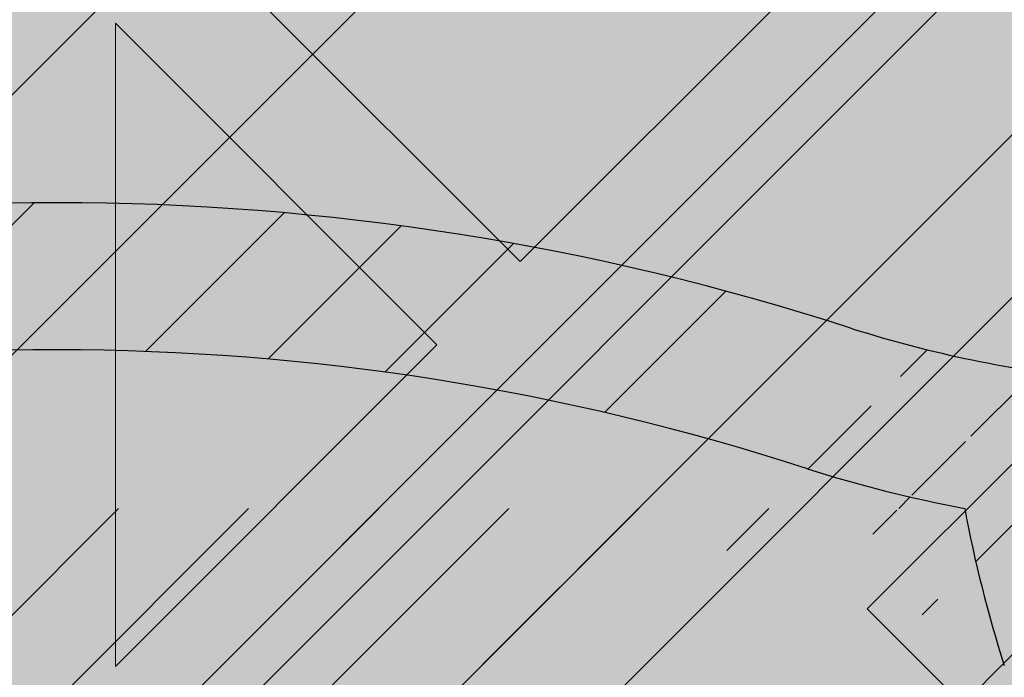
# Model space of a CAD drawing. Units: inches. Extents: x 844 to 2234, y 346 to 1084.
# Tile 20 of 93: x 1122.777 to 1124.911, y 702.178 to 703.603. Entities that reach past the tile are written whole.
import ezdxf

# ---------------------------------------------------------------- set-up
doc = ezdxf.new("R2010")
doc.units = ezdxf.units.IN
doc.header["$MEASUREMENT"] = 0
for name, color, linetype, lineweight in [('A-ANNO-DIMS', 2, 'Continuous', 18), ('furniture', 8, 'Continuous', 18), ('RA-AP-01$0$INT', 35, 'Continuous', 5)]:
    doc.layers.add(name, color=color, linetype=linetype, lineweight=lineweight)
doc.layers.add('RA-AP-01$0$FURN', color=3, linetype='Continuous')
doc.layers.add('RA-AP-01$0$WOOD', color=64, linetype='Continuous')
doc.styles.get("Standard").update_dxf_attribs({"font": 'arial.ttf'})
doc.dimstyles.get("Standard").update_dxf_attribs({"dimtxt": 6, "dimasz": 3, "dimexe": 0.18, "dimexo": 0.0625, "dimgap": 0.09, "dimtad": 0, "dimtih": 1, "dimtoh": 1, "dimdec": 1, "dimzin": 0, "dimdsep": 46, "dimlunit": 3, "dimtxsty": 'Standard', "dimblk": 'ARCHTICK', "dimcen": 0.09, "dimadec": 0, "dimazin": 0, "dimtfac": 1, "dimtdec": 1, "dimtofl": 0, "dimtmove": 0, "dimatfit": 3, "dimfxl": 1, "dimtolj": 1, "dimtzin": 0, "dimarcsym": 0})

# ---------------------------------------------------------------- blocks, each defined once
blk = doc.blocks.new('A$C18D01794')
at = {"layer": 'RA-AP-01$0$INT'}
h = blk.add_hatch(color=256, dxfattribs=at)
h.paths.add_polyline_path([(4.585917135068448, -7.856712009587804), (4.614201406330596, -7.856712009587056), (4.668846067270487, -7.802067348644738), (4.723490728212344, -7.856712009584164), (4.771774999457151, -7.856712009582887), (4.826419660396886, -7.80206734864072), (4.862780050090322, -7.838427738332541), (4.844495778842715, -7.856712009580965), (4.862780050090411, -7.856712009580482), (4.905206456960182, -7.814285602707865), (4.947632863832445, -7.856712009578238), (4.965917135079675, -7.856712009577755), (4.947632863831759, -7.838427738330656), (4.983993253523576, -7.802067348637219), (5.038637914464627, -7.856712009575829), (5.08692218571208, -7.856712009574554), (5.141566846649976, -7.802067348634224), (5.196211507589851, -7.856712009571666), (5.224495778822615, -7.856712009570916), (4.905206456953975, -7.537422687702283)])
h.paths.add_polyline_path([(4.895206456956031, -7.575706958950402), (4.895206456958921, -7.684996280828174), (4.840561796018589, -7.630351619890275)], flags=16)
h.paths.add_polyline_path([(4.915206456955638, -7.575706958949956), (4.969851117895509, -7.630351619887399), (4.915206456957609, -7.684996280827732)], flags=16)
h.paths.add_polyline_path([(4.826419660395175, -7.644493755514321), (4.881064321335613, -7.699138416452331), (4.771774999456703, -7.69913841645522)], flags=16)
h.paths.add_polyline_path([(4.983993253519558, -7.644493755510815), (5.038637914460456, -7.699138416449285), (4.929348592581548, -7.69913841645126)], flags=16)
h.paths.add_polyline_path([(4.881064321336025, -7.719138416452334), (4.826419660397532, -7.773783077393256), (4.771774999457062, -7.719138416455217)], flags=16)
h.paths.add_polyline_path([(4.929348592582019, -7.71913841645126), (5.038637914460982, -7.719138416449284), (4.983993253522945, -7.773783077389749)], flags=16)
h.paths.add_polyline_path([(4.895206456960191, -7.733280552075633), (4.895206456962115, -7.806001331460164), (4.876922185715016, -7.824285602708492), (4.840561796021581, -7.787925213016675)], flags=16)
h.paths.add_polyline_path([(4.915206456958487, -7.733280552075187), (4.969851117899527, -7.787925213013798), (4.933490728206909, -7.824285602708034), (4.9152064569598, -7.806001331461736)], flags=16)
h.paths.add_polyline_path([(4.757632863832376, -7.733280552079264), (4.812277524772842, -7.787925213017304), (4.757632863834348, -7.842569873958233)], flags=16)
h.paths.add_polyline_path([(4.737632863832376, -7.73328055207979), (4.737632863834348, -7.842569873958701), (4.682988202893906, -7.787925213020692)], flags=16)
h.paths.add_polyline_path([(5.05278005008503, -7.733280552072701), (5.052780050087917, -7.842569873951664), (4.998135389146995, -7.787925213013169)], flags=16)
h.paths.add_polyline_path([(5.072780050085024, -7.733280552072333), (5.127424711025931, -7.787925213010806), (5.072780050087916, -7.842569873951244)], flags=16)
h.paths.add_polyline_path([(4.935917135072783, -7.506712009583784), (5.255206456948811, -7.826001331459767), (5.255206456948932, -7.797717060211899), (5.200561796010279, -7.743072399273238), (5.255206456949403, -7.688427738334128), (5.25520645694961, -7.640143467086677), (5.200561796009787, -7.585498806146837), (5.236922185702417, -7.549138416454212), (5.255206456949919, -7.56742268770172), (5.255206456949998, -7.549138416454178), (5.212780050078687, -7.506712009583814), (5.25520645695036, -7.464285602712145), (5.255206456950438, -7.446001331464763), (5.236922185702424, -7.464285602712779), (5.200561796009796, -7.427925213020149), (5.255206456950753, -7.373280552079203), (5.25520645695096, -7.324996280834394), (5.200561796010322, -7.270351619893748), (5.255206456951428, -7.215706958952649), (5.255206456951547, -7.187422687705071)])
h.paths.add_polyline_path([(5.042988202883395, -7.42792521302065), (5.097632863823085, -7.373280552080975), (5.097632863822622, -7.482569873959883)], flags=16)
h.paths.add_polyline_path([(5.028846067259663, -7.442067348644384), (5.083490728198774, -7.496712009583504), (4.974201406321001, -7.496712009583035)], flags=16)
h.paths.add_polyline_path([(5.117632863823087, -7.37328055208089), (5.172277524762331, -7.42792521302015), (5.11763286382262, -7.482569873959851)], flags=16)
h.paths.add_polyline_path([(5.08349072819877, -7.516712009582191), (5.028846067259652, -7.571356670521302), (4.974201406320998, -7.516712009582638)], flags=16)
h.paths.add_polyline_path([(5.131774999446817, -7.35913841645716), (5.186419660386065, -7.413783077396415), (5.241064321325782, -7.359138416456712)], flags=17)
h.paths.add_polyline_path([(5.131774999446228, -7.496712009583703), (5.186419660386065, -7.442067348643883), (5.222780050079488, -7.478427738337313), (5.204495778832781, -7.496712009584014)], flags=16)
h.paths.add_polyline_path([(5.097632863822613, -7.530854145205813), (5.097632863823061, -7.640143467084723), (5.042988202883383, -7.585498806145032)], flags=16)
h.paths.add_polyline_path([(5.131774999446899, -7.339138416457162), (5.241064321325809, -7.339138416456712), (5.186419660386591, -7.284493755517479)], flags=17)
h.paths.add_polyline_path([(5.131774999446226, -7.516712009581999), (5.204495778830767, -7.516712009581702), (5.22278005007868, -7.534996280829206), (5.186419660386049, -7.571356670521828)], flags=16)
h.paths.add_polyline_path([(5.11763286382262, -7.530854145205852), (5.17227752476232, -7.585498806145562), (5.117632863823064, -7.64014346708481)], flags=16)
h.paths.add_polyline_path([(5.186419660386069, -7.599640941770585), (5.241064321325754, -7.654285602710281), (5.131774999446791, -7.654285602709814)], flags=16)
h.paths.add_polyline_path([(5.131774999446872, -7.674285602709813), (5.24106432132578, -7.674285602710282), (5.186419660386554, -7.728930263649504)], flags=16)
h.paths.add_polyline_path([(5.255206456951811, -7.126001331467467), (5.255206456951895, -7.106712009588038), (4.555206456956052, -7.106712009588038), (4.555206456956136, -7.12600133146746), (4.905206456953973, -7.476001331465289)])
h.paths.add_polyline_path([(4.983993253513404, -7.368930263651977), (4.92934859257295, -7.314285602713969), (5.03863791445186, -7.314285602711063)], flags=16)
h.paths.add_polyline_path([(4.969851117889988, -7.383072399276016), (4.915206456952556, -7.437717060215906), (4.915206456949648, -7.328427738338133)], flags=16)
h.paths.add_polyline_path([(4.929348592572535, -7.294285602713971), (4.983993253511019, -7.239640941773039), (5.038637914451496, -7.294285602711065)], flags=16)
h.paths.add_polyline_path([(5.052780050074912, -7.280143467087016), (4.998135389134438, -7.225498806148989), (5.052780050072919, -7.170854145208052)], flags=16)
h.paths.add_polyline_path([(5.07278005007491, -7.280143467086489), (5.072780050072918, -7.170854145207579), (5.127424711013374, -7.225498806145578)], flags=16)
h.paths.add_polyline_path([(4.89520645695295, -7.437717060216355), (4.840561796013067, -7.383072399278919), (4.895206456950961, -7.328427738338582)], flags=16)
h.paths.add_polyline_path([(4.915206456948365, -7.280143467090674), (4.915206456946434, -7.207422687704125), (4.933490728192729, -7.18913841645701), (4.969851117886972, -7.225498806149623)], flags=16)
h.paths.add_polyline_path([(4.881064321327021, -7.314285602715054), (4.82641966038902, -7.368930263655506), (4.771774999448108, -7.314285602717047)], flags=16)
h.paths.add_polyline_path([(4.895206456950073, -7.280143467091125), (4.840561796009022, -7.225498806152518), (4.876922185700835, -7.18913841645908), (4.895206456948749, -7.207422687706589)], flags=16)
h.paths.add_polyline_path([(4.983993253510392, -7.211356670525576), (4.947632863816944, -7.174996280833758), (4.965917135064043, -7.156712009585847), (5.038637914448995, -7.156712009584522)], flags=16)
h.paths.add_polyline_path([(4.881064321326543, -7.294285602715056), (4.771774999447578, -7.294285602717046), (4.826419660385607, -7.239640941776569)], flags=16)
h.paths.add_polyline_path([(4.905206456946447, -7.19913841645844), (4.862780050074785, -7.156712009587725), (4.947632863816685, -7.156712009586302)], flags=16)
h.paths.add_polyline_path([(5.14156684663679, -7.211356670521528), (5.086922185696452, -7.156712009583639), (5.196211507574223, -7.156712009581651)], flags=16)
h.paths.add_polyline_path([(4.8264196603837, -7.211356670529104), (4.771774999442643, -7.156712009590501), (4.8444957788276, -7.156712009588568), (4.862780050075511, -7.17499628083566)], flags=16)
h.paths.add_polyline_path([(4.812277524760289, -7.225498806153156), (4.757632863822258, -7.28014346709363), (4.757632863819352, -7.170854145214669)], flags=16)
h.paths.add_polyline_path([(4.73763286382226, -7.280143467093997), (4.682988202881349, -7.22549880615554), (4.737632863819352, -7.170854145215086)], flags=16)
h.paths.add_polyline_path([(4.723490728195188, -7.156712009591787), (4.668846067257299, -7.211356670532127), (4.614201406317417, -7.156712009594693)], flags=16)
h.paths.add_polyline_path([(4.597632863829262, -7.506712009583814), (4.555206456957951, -7.54913841645418), (4.555206456958029, -7.56742268770172), (4.573490728205535, -7.549138416454212), (4.609851117898167, -7.585498806146839), (4.555206456958338, -7.640143467086675), (4.555206456958546, -7.688427738334125), (4.60985111789767, -7.743072399273238), (4.555206456959015, -7.797717060211899), (4.555206456959138, -7.826001331459767), (4.874495778835167, -7.506712009583786), (4.5552064569564, -7.187422687705062), (4.555206456956523, -7.215706958952644), (4.609851117897629, -7.270351619893746), (4.555206456956988, -7.324996280834396), (4.555206456957198, -7.373280552079195), (4.609851117898153, -7.427925213020147), (4.573490728205528, -7.464285602712779), (4.555206456957507, -7.446001331464756), (4.555206456957585, -7.464285602712143)])
h.paths.add_polyline_path([(4.712780050085332, -7.482569873959882), (4.712780050084863, -7.373280552080972), (4.767424711024555, -7.42792521302065)], flags=16)
h.paths.add_polyline_path([(4.726922185709173, -7.496712009583504), (4.781566846648288, -7.442067348644384), (4.836211507586949, -7.496712009583033)], flags=16)
h.paths.add_polyline_path([(4.692780050085327, -7.482569873959851), (4.638135389145619, -7.427925213020149), (4.692780050084865, -7.373280552080892)], flags=16)
h.paths.add_polyline_path([(4.726922185709182, -7.516712009582191), (4.836211507586949, -7.51671200958264), (4.7815668466483, -7.571356670521304)], flags=16)
h.paths.add_polyline_path([(4.678637914461726, -7.496712009583706), (4.605917135075169, -7.496712009584014), (4.587632863828464, -7.478427738337311), (4.623993253521887, -7.442067348643881)], flags=16)
h.paths.add_polyline_path([(4.712780050085336, -7.530854145205816), (4.767424711024568, -7.585498806145034), (4.71278005008489, -7.640143467084724)], flags=16)
h.paths.add_polyline_path([(4.678637914461726, -7.516712009582001), (4.623993253521899, -7.571356670521829), (4.587632863829271, -7.534996280829206), (4.605917135077185, -7.5167120095817)], flags=16)
h.paths.add_polyline_path([(4.692780050085336, -7.530854145205848), (4.692780050084889, -7.64014346708481), (4.638135389145632, -7.585498806145562)], flags=16)
h.paths.add_polyline_path([(4.623993253521885, -7.413783077396415), (4.678637914461131, -7.359138416457161), (4.56934859258217, -7.359138416456712)], flags=17)
h.paths.add_polyline_path([(4.623993253521901, -7.599640941770568), (4.678637914461158, -7.654285602709814), (4.569348592582195, -7.654285602710281)], flags=16)
h.paths.add_polyline_path([(4.678637914461051, -7.339138416457162), (4.623993253521361, -7.284493755517479), (4.569348592582143, -7.339138416456712)], flags=17)
h.paths.add_polyline_path([(4.678637914461076, -7.674285602709813), (4.623993253521399, -7.728930263649504), (4.569348592582167, -7.674285602710281)], flags=16)
h = blk.add_hatch(color=256, dxfattribs=at)
h.paths.add_polyline_path([(4.905206456954232, -7.537422687702028), (4.874495778835232, -7.506712009583718), (4.555206456959138, -7.826001331459766), (4.555206456959269, -7.856712009588616), (4.585917135068449, -7.856712009587804)])
h.paths.add_polyline_path([(4.935917135072152, -7.506712009583152), (4.905206456953497, -7.537422687701806), (5.224495778822614, -7.856712009570917), (5.255206456948681, -7.856712009570104), (5.255206456948813, -7.826001331459768)])
h.paths.add_polyline_path([(5.255206456951549, -7.18742268770507), (5.255206456951813, -7.126001331467461), (4.905206456953563, -7.476001331465701), (4.935917135072559, -7.506712009584006)])
h.paths.add_polyline_path([(4.874495778835167, -7.506712009583785), (4.905206456953818, -7.476001331465132), (4.555206456956135, -7.126001331467458), (4.555206456956399, -7.187422687705064)])
h = blk.add_hatch(color=256, dxfattribs=at)
h.paths.add_polyline_path([(5.028846067259997, -7.571356670520955), (4.974201406321342, -7.516712009582294), (5.083490728199115, -7.516712009581846)])
h.paths.add_polyline_path([(4.974201406321344, -7.496712009582688), (5.028846067260004, -7.442067348644037), (5.083490728199117, -7.496712009583157)])
h.paths.add_polyline_path([(5.042988202883738, -7.427925213020309), (5.097632863823428, -7.373280552080627), (5.097632863822963, -7.482569873959537)])
h.paths.add_polyline_path([(5.117632863822961, -7.482569873959509), (5.117632863823428, -7.373280552080546), (5.172277524762674, -7.427925213019804)])
h.paths.add_polyline_path([(5.131774999446572, -7.496712009583358), (5.186419660386406, -7.442067348643536), (5.222780050079831, -7.478427738336961), (5.204495778833122, -7.496712009583667)])
h.paths.add_polyline_path([(5.236922185702764, -7.464285602712433), (5.200561796010139, -7.427925213019802), (5.255206456949971, -7.373280552079975), (5.255206456950271, -7.446001331464927)])
h.paths.add_polyline_path([(5.186419660386412, -7.41378307739607), (5.131774999447164, -7.359138416456815), (5.241064321326123, -7.359138416456366)])
h.paths.add_polyline_path([(5.131774999447238, -7.339138416456815), (5.186419660386934, -7.284493755517132), (5.241064321326153, -7.339138416456368)])
h.paths.add_polyline_path([(5.200561796010663, -7.270351619893402), (5.255206456949324, -7.215706958954747), (5.255206456949777, -7.324996280832518)])
h.paths.add_polyline_path([(5.21278005007903, -7.50671200958347), (5.255206456950223, -7.464285602712278), (5.255206456950696, -7.549138416454185)])
h.paths.add_polyline_path([(5.13177499944657, -7.516712009581652), (5.204495778831106, -7.516712009581354), (5.222780050079024, -7.534996280828858), (5.186419660386397, -7.571356670521485)])
h.paths.add_polyline_path([(5.117632863823405, -7.640143467084465), (5.117632863822955, -7.530854145205498), (5.172277524762665, -7.585498806145217)])
h.paths.add_polyline_path([(5.042988202883727, -7.585498806144689), (5.097632863822957, -7.530854145205474), (5.097632863823407, -7.64014346708438)])
h.paths.add_polyline_path([(5.131774999447135, -7.654285602709467), (5.186419660386394, -7.599640941770219), (5.241064321326097, -7.654285602709933)])
h.paths.add_polyline_path([(5.200561796010128, -7.585498806146492), (5.236922185702758, -7.549138416453866), (5.255206456950264, -7.567422687701371), (5.255206456949948, -7.640143467086325)])
h.paths.add_polyline_path([(5.186419660386895, -7.728930263649157), (5.131774999447213, -7.674285602709467), (5.241064321326127, -7.674285602709934)])
h.paths.add_polyline_path([(5.200561796010624, -7.743072399272893), (5.255206456949745, -7.688427738333778), (5.255206456949276, -7.797717060211553)])
h = blk.add_hatch(color=256, dxfattribs=at)
h.paths.add_polyline_path([(4.969851117891331, -7.630351619889621), (4.915206456952669, -7.575706958950966), (4.915206456952222, -7.684996280828739)])
h.paths.add_polyline_path([(4.895206456953064, -7.575706958950968), (4.840561796014413, -7.630351619889628), (4.895206456953533, -7.684996280828741)])
h.paths.add_polyline_path([(4.826419660390684, -7.644493755513362), (4.771774999451003, -7.699138416453052), (4.881064321329913, -7.699138416452587)])
h.paths.add_polyline_path([(4.881064321329884, -7.719138416452585), (4.771774999450921, -7.719138416453052), (4.82641966039018, -7.773783077392298)])
h.paths.add_polyline_path([(4.895206456953734, -7.733280552076196), (4.840561796013912, -7.787925213016031), (4.876922185707337, -7.824285602709455), (4.895206456954043, -7.806001331462747)])
h.paths.add_polyline_path([(4.862780050082808, -7.838427738332388), (4.826419660390178, -7.802067348639763), (4.771774999450351, -7.856712009579595), (4.844495778835303, -7.856712009579895)])
h.paths.add_polyline_path([(4.812277524766446, -7.787925213016036), (4.757632863827191, -7.733280552076788), (4.757632863826741, -7.842569873955747)])
h.paths.add_polyline_path([(4.737632863827191, -7.733280552076863), (4.682988202887508, -7.787925213016558), (4.737632863826743, -7.842569873955778)])
h.paths.add_polyline_path([(4.668846067263777, -7.802067348640287), (4.614201406325123, -7.856712009578949), (4.723490728202894, -7.856712009579402)])
h.paths.add_polyline_path([(4.905206456953846, -7.814285602708654), (4.862780050082654, -7.856712009579847), (4.947632863824561, -7.85671200958032)])
h.paths.add_polyline_path([(4.915206456952028, -7.733280552076195), (4.91520645695173, -7.806001331460731), (4.933490728199234, -7.824285602708648), (4.96985111789186, -7.787925213016022)])
h.paths.add_polyline_path([(5.038637914454841, -7.719138416453029), (4.929348592575874, -7.71913841645258), (4.983993253515593, -7.773783077392289)])
h.paths.add_polyline_path([(4.983993253515065, -7.644493755513352), (4.929348592575849, -7.699138416452582), (5.038637914454755, -7.699138416453031)])
h.paths.add_polyline_path([(5.052780050079843, -7.73328055207676), (4.998135389140595, -7.787925213016018), (5.052780050080309, -7.842569873955721)])
h.paths.add_polyline_path([(4.983993253516868, -7.802067348639752), (4.947632863824241, -7.838427738332383), (4.965917135071747, -7.856712009579888), (5.038637914456701, -7.856712009579572)])
h.paths.add_polyline_path([(5.127424711019533, -7.787925213016519), (5.072780050079843, -7.733280552076838), (5.07278005008031, -7.842569873955751)])
h.paths.add_polyline_path([(5.141566846643269, -7.802067348640248), (5.086922185704154, -7.85671200957937), (5.196211507581929, -7.856712009578901)])
for p, q in [((4.935917135072783, -7.506712009583784), (5.255206456948813, -7.826001331459769)), ((5.097632863822615, -7.530854145205815), (5.042988202883383, -7.585498806145034)), ((4.905206456953975, -7.537422687702283), (5.224495778822613, -7.856712009570916)), ((4.915206456955636, -7.575706958949957), (4.969851117895507, -7.630351619887399)), ((4.915206456957609, -7.684996280827729), (4.915206456955636, -7.575706958949957)), ((5.042988202883385, -7.585498806145036), (5.097632863823062, -7.640143467084724)), ((4.915206456957613, -7.684996280827727), (4.969851117895507, -7.630351619887399)), ((4.929348592581546, -7.69913841645126), (4.983993253519556, -7.644493755510815)), ((4.983993253519558, -7.644493755510817), (5.038637914460456, -7.699138416449285))]:
    blk.add_line(p, q, dxfattribs=at)
blk = doc.blocks.new('A$C32926AE1')
at = {"layer": 'RA-AP-01$0$FURN'}
h = blk.add_hatch(dxfattribs=at)
h.set_pattern_fill('ANSI31', color=256, scale=0.1, style=0)
h.set_pattern_definition([(45, (0, 0), (-0.0088388347648318, 0.0088388347648318), [])])
edge = h.paths.add_edge_path(flags=16)
edge.add_arc((4.904771284329206, 4.246793130718756), 0.2603971832811541, 75.22398030683196, 104.7760196931204)
edge.add_arc((4.904771284329206, 4.246793130718756), 0.2603971832811541, 75.223980306832, 104.77601969312039, ccw=False)
edge = h.paths.add_edge_path(flags=16)
edge.add_arc((4.904771284329206, 4.067062675376612), 0.2603971832811541, 255.2239803068796, 284.776019693168)
edge.add_arc((4.904771284329206, 4.067062675376612), 0.2603971832811541, 255.22398030687958, 284.77601969316805, ccw=False)
edge = h.paths.add_edge_path(flags=0)
edge.add_arc((4.904771284329206, 4.067062675376612), 0.2603971832811541, 255.2239803068796, 284.776019693168)
edge.add_arc((4.904771284329206, 4.067062675376612), 0.2603971832811541, 255.22398030687958, 284.77601969316805, ccw=False)
edge = h.paths.add_edge_path(flags=0)
edge.add_arc((4.904771284329206, 4.067062675376612), 0.2603971832811541, 255.2239803068796, 284.776019693168)
edge.add_arc((4.904771284329206, 4.067062675376612), 0.2603971832811541, 255.22398030687958, 284.77601969316805, ccw=False)
edge = h.paths.add_edge_path()
edge.add_arc((4.604388392048174, 4.588829985554312), 0.1599999999999918, 342.3781640246255, 354.4317409793762)
edge.add_arc((5.090145208887507, 4.43216705527679), 0.3503971832811637, 162.0091218307731, 180.3186872093483)
edge.add_arc((5.205154176610243, 4.588829985554953), 0.1599999999999917, 185.5682590208461, 197.6218359767349)
edge.add_arc((4.904771284329229, 4.246793130718735), 0.3503971832811761, 72.00912183053516, 107.9908781690354)
edge.add_arc((9.535952835716557, 4.28682295566602), 4.798342501046485, 178.2875002453811, 181.5576802719453)
edge.add_arc((4.719397359771122, 4.43216705527679), 0.3503971832811637, 359.6813127906516, 377.9908781692269)
edge.add_arc((9.535967292294904, 4.286822350292874), 4.778371420254705, 178.2965938931842, 181.5667745797229)
edge.add_arc((4.719397359771122, 4.43216705527679), 0.3303971832811637, 359.6813127906516, 377.9908781692269)
edge.add_arc((0.2735752763637294, 4.286822350292874), 4.7783714202547, 358.4332254202771, 361.7034061068158)
edge.add_arc((5.061434214606998, 4.732549947558029), 0.1600000000000254, 252.3781640250584, 264.4317409792362)
edge.add_arc((4.748108354051257, 4.732549947558012), 0.1600000000000541, 275.5682590208426, 287.6218359759532)
edge.add_arc((4.604388392048115, 4.588829985554317), 0.1800000000000505, 342.3567572500182, 349.3735009646207)
edge.add_arc((5.205154176610254, 4.588829985554976), 0.1800000000000069, 190.6264990356027, 197.6432427513933)
edge.add_arc((5.061434214607106, 4.732549947558013), 0.1800000000000424, 252.3567572496606, 259.3735009644582)
edge.add_arc((4.904771284329208, 4.246793130718737), 0.3303971832811676, 71.99844483668534, 108.0015551637021)
edge.add_arc((4.748108354051414, 4.732549947558045), 0.1800000000000547, 280.6264990355479, 287.6432427495938)
edge.add_arc((5.090145208887514, 4.432167055276789), 0.2803971832811691, 162.8706300666893, 180.816523289902)
edge.add_arc((4.719397359771136, 4.432167055276689), 0.2803971832811534, 359.183476710103, 377.1293699333214)
edge.add_arc((4.904771284329222, 4.246793130718737), 0.2803971832811769, 72.87063006672916, 107.1293699332334)
edge.add_arc((5.090145208887522, 4.432167055276788), 0.2603971832811776, 165.2239803068007, 180.9953123810312)
edge.add_arc((4.719397359771141, 4.432167055276699), 0.2603971832811458, 359.0046876189768, 374.7760196932087)
edge.add_arc((5.090145208887507, 4.43216705527679), 0.3303971832811637, 162.0091218307731, 180.3186872093483)
edge.add_arc((9.53595427642584, 4.285015535491528), 4.728345371032053, 178.265043920078, 181.5679956281801)
edge.add_arc((0.2735882922327999, 4.285015535491582), 4.728345371032045, 358.4320043718193, 361.7349560799204)
edge.add_arc((9.535953591267507, 4.284458026472751), 4.708343996644348, 178.2573054306777, 181.5704995759608)
edge.add_arc((0.273588977391114, 4.284458026472785), 4.708343996644358, 358.4295004240388, 361.7426945693213)
edge.add_arc((0.2735889773911131, 4.029397779622582), 4.708343996644359, 358.2573054306787, 361.5704995759613)
edge.add_arc((9.535953591267518, 4.029397779622618), 4.708343996644359, 178.4295004240391, 181.7426945693223)
edge.add_arc((0.2735882922327901, 4.028840270603786), 4.728345371032054, 358.2650439200796, 361.5679956281808)
edge.add_arc((9.53595427642584, 4.028840270603841), 4.728345371032054, 178.4320043718199, 181.7349560799219)
edge.add_arc((0.2735752763637302, 4.027033455802493), 4.778371420254699, 358.2965938931842, 361.5667745797229)
edge.add_arc((4.719397359771122, 3.881688750818578), 0.3303971832811637, 342.0091218307731, 360.3186872093484)
edge.add_arc((5.090145208887507, 3.881688750818578), 0.3303971832811637, 179.6813127906516, 197.9908781692269)
edge.add_arc((9.535967292294904, 4.027033455802493), 4.778371420254705, 178.433225420277, 181.7034061068158)
edge.add_arc((4.719397359771122, 3.881688750818578), 0.3503971832811637, 342.0091218307731, 360.3186872093484)
edge.add_arc((9.53595283571655, 4.027032850429349), 4.79834250104648, 178.4423197280546, 181.7124997546188)
edge.add_arc((4.719397359771141, 3.881688750818669), 0.2603971832811458, 345.2239803067913, 360.9953123810232)
edge.add_arc((5.090145208887522, 3.88168875081858), 0.2603971832811776, 179.0046876189687, 194.7760196931993)
edge.add_arc((4.904771284329222, 4.067062675376631), 0.2803971832811769, 252.8706300667665, 287.1293699332708)
edge.add_arc((4.719397359771136, 3.881688750818678), 0.2803971832811534, 342.8706300666787, 360.8165232898969)
edge.add_arc((5.090145208887514, 3.881688750818579), 0.2803971832811691, 179.183476710098, 197.1293699333106)
edge.add_arc((4.748108354051414, 3.581305858537323), 0.1800000000000547, 72.3567572504062, 79.37350096445199)
edge.add_arc((4.904771284329208, 4.067062675376631), 0.3303971832811676, 251.9984448362979, 288.0015551633146)
edge.add_arc((5.061434214607106, 3.581305858537355), 0.1800000000000424, 100.6264990355418, 107.6432427503394)
edge.add_arc((5.205154176610254, 3.725025820540392), 0.1800000000000069, 162.3567572486066, 169.3735009643972)
edge.add_arc((4.604388392048115, 3.725025820541051), 0.1800000000000505, 10.62649903537925, 17.64324274998182)
edge.add_arc((4.748108354051257, 3.581305858537356), 0.1600000000000541, 72.37816402404681, 84.43174097915735)
edge.add_arc((4.904771284329229, 4.067062675376632), 0.3503971832811761, 252.0091218309645, 287.9908781694648)
edge.add_arc((5.061434214606998, 3.581305858537339), 0.1600000000000254, 95.56825902076373, 107.6218359749416)
edge.add_arc((5.205154176610243, 3.725025820540414), 0.1599999999999917, 162.3781640232651, 174.4317409791539)
edge.add_arc((5.090145208887507, 3.881688750818578), 0.3503971832811637, 179.6813127906516, 197.9908781692269)
edge.add_arc((4.604388392048174, 3.725025820541056), 0.1599999999999918, 5.568259020623824, 17.62183597537444)
edge.add_arc((0.2735897329420762, 4.28682295566602), 4.798342501046482, 358.4423197280547, 361.7124997546188)
edge.add_arc((0.2735897329420691, 4.027032850429348), 4.798342501046489, 358.2875002453812, 361.5576802719453)
at = {"layer": 'RA-AP-01$0$WOOD'}
h = blk.add_hatch(color=256, dxfattribs=at)
h.dxf.hatch_style = 1
h.paths.add_polyline_path([(5.157430609644524, 4.573483066760929, -0.1009492694046607), (5.155401577623758, 4.593365984175333, -0.1842662638101597), (5.172249623284174, 4.638795604568598, 0.2056608120311276), (5.179560981299304, 4.661316324430096, 0.3614336704623542), (5.134352340494423, 4.706524965234944, 0.2056608120311297), (5.111831620632933, 4.699213607219793, -0.1842662638101113), (5.066402000239693, 4.682365561559342, -0.1055311479399994), (5.045656153913092, 4.68467289944697, 0.1567636581983829), (4.763886414745334, 4.684672899446966, -0.1055311479399895), (4.743140568418733, 4.68236556155934, -0.1842662638100833), (4.6977109480255, 4.69921360721979, 0.2056608120302612), (4.675190228164109, 4.706524965234949, 0.3614336704708441), (4.629981587358889, 4.66131632442871, 0.2056608120245944), (4.637292945374126, 4.638795604567974, -0.1842662638101024), (4.654140991034615, 4.59336598417475, -0.1009492694055169), (4.652111959013835, 4.573483066760181, 0.021410119221476), (4.629748025606143, 4.156712009541676, 0.0214101192214795), (4.652111959013809, 3.739940952323101, -0.1009492694059586), (4.654140991034615, 3.720058034908448, -0.1842662638100975), (4.637292945374126, 3.674628414515226, 0.2056608120245705), (4.629981587358889, 3.652107694654492, 0.3614336704708879), (4.675190228164113, 3.606899053848249, 0.2056608120302384), (4.697710948025501, 3.614210411863408, -0.1842662638100995), (4.743140568418738, 3.63105845752386, -0.1055311479402541), (4.763886414745388, 3.628751119636215, 0.1567636581983776), (5.045656153913137, 3.628751119636244, -0.1055311479397538), (5.066402000239692, 3.631058457523857, -0.1842662638101067), (5.111831620632931, 3.614210411863407, 0.2056608120310924), (5.134352340494417, 3.606899053848256, 0.3614336704624001), (5.179560981299307, 3.652107694653103, 0.2056608120311314), (5.172249623284175, 3.6746284145146, -0.1842662638101402), (5.155401577623758, 3.72005803490786, -0.1009492694051366), (5.15743060964455, 3.739940952322354, 0.0214101192215073), (5.179794543052287, 4.156712009541468, 0.0214101192215252)])
h.paths.add_polyline_path([(4.639748609479751, 4.156712009541513, 0.0213537860821624), (4.661970494867118, 3.741887061152232, -0.094075836301374), (4.664143710413708, 3.7196126951003, -0.1824818158568985), (4.644813765429836, 3.668037719127816, 0.2056608120245319), (4.639939526753007, 3.653023905887301, 0.3614336704710246), (4.676106439397173, 3.616856993242342, 0.2056608120302234), (4.691120252638095, 3.621731231919122, -0.1824818158602558), (4.742695228611606, 3.641061176902986, -0.1029891339458722), (4.766991894714349, 3.638256818950944, 0.156709409989566), (5.042550673941472, 3.638256818950105, -0.102989133958497), (5.066847340047078, 3.641061176902949, -0.1824818158594995), (5.118422316020358, 3.621731231919103, 0.2056608120311416), (5.133436129261316, 3.616856993242346, 0.3614336704621468), (5.169603041905217, 3.653023905886178, 0.2056608120310986), (5.164728803228477, 3.668037719127177, -0.1824818158565612), (5.145398858244737, 3.719612695099578, -0.0940758363009313), (5.147572073791232, 3.741887061151398, 0.0213537860822023), (5.169793959178681, 4.156712009541451, 0.0213537860822226), (5.147572073791203, 4.571536957931898, -0.0940758363005034), (5.145398858244737, 4.59381132398362, -0.1824818158565587), (5.164728803228476, 4.645386299956021, 0.2056608120311045), (5.169603041905216, 4.66040011319702, 0.3614336704621845), (5.133436129261313, 4.696567025840856, 0.2056608120310773), (5.118422316020359, 4.691692787164098, -0.182481815859508), (5.066847340047078, 4.67236284218025, -0.1029891339584606), (5.04255067394148, 4.675167200133092, 0.156709409989566), (4.766991894714357, 4.675167200132257, -0.1029891339458842), (4.742695228611611, 4.672362842180213, -0.1824818158602725), (4.691120252638095, 4.691692787164077, 0.2056608120302152), (4.676106439397174, 4.696567025840858, 0.3614336704710363), (4.639939526753005, 4.660400113195899, 0.2056608120245495), (4.644813765429837, 4.645386299955384, -0.1824818158568934), (4.664143710413708, 4.593811323982902, -0.0940758363009187), (4.661970494867149, 4.571536957931074, 0.021353786082177)], flags=16)
h.paths.add_polyline_path([(5.129794543052235, 4.432167055276933, -0.0141661062790638), (5.130152669293814, 4.156927903047693, -0.0141661062790647), (5.129794543052234, 3.881688750818433, -0.0785247771143638), (5.10979738006795, 3.755143611847103, 0.0945969212073497), (5.105408519571111, 3.717898134952927, 0.1043170707844957), (5.116074640131521, 3.670385395016088, 0.1043170707864965), (5.068561900193738, 3.681051515576561, 0.09459692119553), (5.031316423304057, 3.676662655080835, -0.1580239521427272), (4.778226145355827, 3.676662655080367, 0.0945969211986668), (4.740980668464973, 3.681051515576592, 0.1043170707882822), (4.693467928526415, 3.670385395015844, 0.1043170707867916), (4.704134049087309, 3.717898134953662, 0.0945969211972894), (4.69974518859162, 3.755143611844042, -0.0785247771163196), (4.679748025606343, 3.881688750818406, -0.0141661062790663), (4.679389899364763, 4.156927903047693, -0.0141661062790672), (4.679748025606343, 4.432167055276998, -0.0785247771163064), (4.699745188591625, 4.55871219425134, 0.094596921197333), (4.704134049087308, 4.595957671141738, 0.1043170707867205), (4.693467928526416, 4.643470411079523, 0.1043170707882628), (4.740980668464965, 4.632804290518776, 0.0945969211988114), (4.778226145355874, 4.637193151015016, -0.158023952142669), (5.031316423304015, 4.637193151014546, 0.0945969211956361), (5.068561900193736, 4.632804290518806, 0.1043170707864979), (5.11607464013152, 4.643470411079278, 0.1043170707844617), (5.105408519571112, 4.595957671142455, 0.0945969212074597), (5.109797380067959, 4.558712194248236, -0.0785247771143467)], flags=0)
h.paths.add_polyline_path([(5.119794532311105, 4.432259799204851, -0.0142000800617244), (5.120156169157484, 4.156927903047701, -0.0142000800617277), (5.119794532311105, 3.881596006890482, -0.0784894509520253), (5.100273383573699, 3.758192358677797, 0.0940138827242913), (5.095413455884425, 3.717477693979438, 0.0606271852308753), (5.099615656341024, 3.686844378806616, 0.0606271852322524), (5.068982341167493, 3.691046579263239, 0.0940138827010453), (5.028267676478798, 3.686186651576848, -0.1580706864508061), (4.781274892180912, 3.686186651576435, 0.0940138827026903), (4.740560227491556, 3.691046579263279, 0.0606271852339895), (4.709926912317155, 3.686844378806508, 0.0606271852329405), (4.714129112773991, 3.717477693980356, 0.094013882701304), (4.709269185087677, 3.758192358669163, -0.0784894509577193), (4.689748036347473, 3.881596006890469, -0.014200080061729), (4.689386399501094, 4.156927903047709, -0.0142000800617217), (4.689748036347473, 4.432259799204808, -0.078489450957724), (4.709269185087651, 4.555663447426125, 0.0940138827014585), (4.714129112773992, 4.596378112114996, 0.0606271852329731), (4.709926912317154, 4.62701142728886, 0.0606271852340196), (4.74056022749157, 4.622809226832087, 0.0940138827024997), (4.781274892180847, 4.627669154518912, -0.1580706864508359), (5.028267676478777, 4.627669154518526, 0.0940138827010946), (5.068982341167492, 4.622809226832129, 0.060627185232254), (5.099615656341024, 4.627011427288751, 0.0606271852308727), (5.095413455884425, 4.59637811211593, 0.0940138827241088), (5.100273383573675, 4.555663447417647, -0.0784894509520978)], flags=0)
h.paths.add_polyline_path([(5.06978912287499, 4.430218106756144, -0.014241683694547), (5.070173729147532, 4.156927903047672, -0.0142416836945458), (5.06978912287499, 3.883637699339223, -0.0800609523125196), (5.052662118612511, 3.773463122773442, 0.0526421978001116), (5.04590916754064, 3.740550867606997, 0.0526421977992423), (5.012996912374707, 3.73379791653534, -0.1583028414718258), (4.796545656286308, 3.73379791653451, 0.0526421978034211), (4.763633401117837, 3.740550867607021, 0.0526421978018622), (4.756880450045755, 3.773463122774558, -0.0800609523117106), (4.739753445783639, 3.883637699339268, -0.0142416836945435), (4.739368839511098, 4.156927903047671, -0.0142416836945477), (4.739753445783639, 4.430218106756155, -0.0800609523116345), (4.75688045004574, 4.540392683320762, 0.052642197801941), (4.763633401117837, 4.573304938488346, 0.0526421978035071), (4.796545656286361, 4.580057889560873, -0.1583028414717561), (5.012996912374669, 4.580057889560039, 0.0526421977993048), (5.04590916754064, 4.57330493848837, 0.0526421978002057), (5.052662118612529, 4.540392683321868, -0.080060952312477)], flags=0)
h.paths.add_polyline_path([(5.049789715110557, 4.43038092723357, -0.0143097550741839), (5.05018085590259, 4.156927903047715, -0.0143097550741854), (5.049789715110558, 3.883474878861827, -0.0800685599149176), (5.03362098255317, 3.779581877367999, 0.0306258898956367), (5.028241146483733, 3.758218888663947, 0.0306258898977031), (5.006878157778253, 3.75283905259408, -0.1583983521624096), (4.802664410878162, 3.752839052594731, 0.0306258898946014), (4.781301422174808, 3.758218888663924, 0.0306258898967912), (4.775921586105202, 3.779581877368794, -0.080068559914251), (4.759752853548071, 3.883474878861786, -0.0143097550741854), (4.759361712756037, 4.156927903047671, -0.0143097550741854), (4.759752853548071, 4.430380927233557, -0.0800685599142479), (4.775921586105193, 4.534273928726546, 0.0306258898968306), (4.781301422174808, 4.555636917431444, 0.0306258898945754), (4.802664410878143, 4.561016753500631, -0.1583983521624168), (5.006878157778244, 4.561016753501291, 0.0306258898977177), (5.028241146483733, 4.555636917431421, 0.0306258898958182), (5.03362098255321, 4.534273928727244, -0.080068559914796)], flags=0)
h.paths.add_polyline_path([(4.999766070382627, 4.428171244713864, -0.0143443147609634), (5.000198441819402, 4.156927903047689, -0.0143443147609612), (4.999766070382627, 3.885684561381556, -0.0784641635803329), (4.987356730658798, 3.799103304488872, -0.1506053783831347), (4.822185837999821, 3.79910330448882, -0.0784641635803318), (4.809776498276007, 3.885684561381509, -0.014344314760963), (4.809344126839227, 4.156927903047677, -0.0143443147609645), (4.809776498276007, 4.428171244713873, -0.0784641635803192), (4.822185837999822, 4.514752501606549, -0.1506053783831338), (4.987356730658798, 4.514752501606494, -0.078464163580285)], flags=0)
h.paths.add_polyline_path([(4.979755254238824, 4.42764379880488, -0.0143772539198268), (4.980205517789977, 4.156927903047693, -0.0143772539198275), (4.979755254238824, 3.886212007290489, -0.0689242507424422), (4.971183264704897, 3.815276770442801, -0.1296645318904179), (4.838359303953726, 3.815276770442746, -0.0689242507424186), (4.829787314419809, 3.886212007290419, -0.0143772539198292), (4.829337050868653, 4.156927903047653, -0.0143772539198325), (4.829787314419809, 4.427643798804946, -0.0689242507424211), (4.838359303953725, 4.498579035652621, -0.1296645318904187), (4.971183264704897, 4.498579035652565, -0.0689242507424401)], flags=0)
h = blk.add_hatch(color=256, dxfattribs=at)
h.dxf.hatch_style = 1
h.paths.add_polyline_path([(5.145398858244737, 4.59381132398362, -0.1824818158565616), (5.164728803228476, 4.645386299956021, 0.2056608120311045), (5.169603041905216, 4.66040011319702, 0.3614336704621845), (5.133436129261313, 4.696567025840856, 0.2056608120310773), (5.118422316020359, 4.691692787164098, -0.182481815859508), (5.066847340047078, 4.67236284218025, -0.1029891339584606), (5.04255067394148, 4.675167200133092, 0.156709409989566), (4.766991894714357, 4.675167200132257, -0.1029891339458842), (4.742695228611611, 4.672362842180213, -0.1824818158602725), (4.691120252638095, 4.691692787164077, 0.2056608120302152), (4.676106439397174, 4.696567025840858, 0.3614336704710363), (4.639939526753005, 4.660400113195899, 0.2056608120245495), (4.644813765429837, 4.645386299955384, -0.1824818158568934), (4.664143710413708, 4.593811323982902, -0.0940758363009187), (4.661970494867149, 4.571536957931074, 0.0213537860821772), (4.639748609479751, 4.156712009541507, 0.0213537860821625), (4.661970494867119, 3.741887061152226, -0.0940758363013071), (4.664143710413708, 3.719612695100309, -0.1824818158569294), (4.644813765429836, 3.668037719127816, 0.2056608120245319), (4.639939526753007, 3.653023905887301, 0.3614336704710246), (4.676106439397173, 3.616856993242342, 0.2056608120302234), (4.691120252638095, 3.621731231919122, -0.1824818158602558), (4.742695228611606, 3.641061176902986, -0.1029891339458722), (4.766991894714349, 3.638256818950944, 0.156709409989566), (5.042550673941472, 3.638256818950105, -0.102989133958497), (5.066847340047078, 3.641061176902949, -0.1824818158594995), (5.118422316020358, 3.621731231919103, 0.2056608120311416), (5.133436129261316, 3.616856993242346, 0.3614336704621468), (5.169603041905217, 3.653023905886178, 0.2056608120310986), (5.164728803228477, 3.668037719127177, -0.1824818158565612), (5.145398858244737, 3.719612695099578, -0.0940758363009313), (5.147572073791232, 3.741887061151398, 0.0213537860822023), (5.169793959178681, 4.156712009541451, 0.0213537860822226), (5.147572073791203, 4.571536957931898, -0.0940758363004996)])
h.paths.add_polyline_path([(5.109797380067958, 4.55871219424824, -0.0785247771143472), (5.129794543052234, 4.432167055276936, -0.0141661062790644), (5.130152669293814, 4.156927903047685, -0.014166106279066), (5.129794543052234, 3.881688750818401, -0.0785247771143517), (5.109797380067946, 3.755143611847092, 0.0945969212073132), (5.105408519571111, 3.717898134952929, 0.1043170707844995), (5.116074640131521, 3.670385395016088, 0.1043170707864965), (5.068561900193738, 3.681051515576561, 0.09459692119553), (5.031316423304057, 3.676662655080835, -0.1580239521427272), (4.778226145355827, 3.676662655080367, 0.0945969211986668), (4.740980668464973, 3.681051515576592, 0.1043170707882822), (4.693467928526415, 3.670385395015844, 0.1043170707867916), (4.704134049087309, 3.717898134953662, 0.0945969211972894), (4.69974518859162, 3.755143611844042, -0.0785247771163196), (4.679748025606343, 3.881688750818406, -0.0141661062790663), (4.679389899364763, 4.156927903047693, -0.0141661062790672), (4.679748025606343, 4.432167055276998, -0.0785247771163064), (4.699745188591625, 4.55871219425134, 0.094596921197333), (4.704134049087308, 4.595957671141738, 0.1043170707867205), (4.693467928526416, 4.643470411079523, 0.1043170707882628), (4.740980668464965, 4.632804290518776, 0.0945969211988114), (4.778226145355874, 4.637193151015016, -0.158023952142669), (5.031316423304015, 4.637193151014546, 0.0945969211956361), (5.068561900193736, 4.632804290518806, 0.1043170707864979), (5.11607464013152, 4.643470411079278, 0.1043170707844617), (5.105408519571112, 4.595957671142455, 0.0945969212074504)], flags=16)
h.paths.add_polyline_path([(5.100273383573655, 4.55566344741771, -0.0784894509521388), (5.119794532311105, 4.432259799204852, -0.0142000800617252), (5.120156169157484, 4.156927903047686, -0.014200080061726), (5.119794532311105, 3.881596006890502, -0.0784894509520446), (5.100273383573696, 3.758192358677786, 0.0940138827242721), (5.095413455884425, 3.717477693979436, 0.0606271852308692), (5.099615656341024, 3.686844378806616, 0.0606271852322522), (5.068982341167493, 3.691046579263239, 0.0940138827010453), (5.028267676478798, 3.686186651576848, -0.1580706864508061), (4.781274892180912, 3.686186651576435, 0.0940138827026903), (4.740560227491556, 3.691046579263279, 0.0606271852339895), (4.709926912317155, 3.686844378806508, 0.0606271852329405), (4.714129112773991, 3.717477693980356, 0.094013882701304), (4.709269185087677, 3.758192358669163, -0.0784894509577193), (4.689748036347473, 3.881596006890469, -0.014200080061729), (4.689386399501094, 4.156927903047709, -0.0142000800617217), (4.689748036347473, 4.432259799204808, -0.078489450957724), (4.709269185087651, 4.555663447426125, 0.0940138827014585), (4.714129112773992, 4.596378112114996, 0.0606271852329731), (4.709926912317154, 4.62701142728886, 0.0606271852340196), (4.74056022749157, 4.622809226832087, 0.0940138827024997), (4.781274892180847, 4.627669154518912, -0.1580706864508359), (5.028267676478777, 4.627669154518526, 0.0940138827010946), (5.068982341167492, 4.622809226832129, 0.060627185232254), (5.099615656341024, 4.627011427288751, 0.0606271852308727), (5.095413455884425, 4.59637811211593, 0.094013882723957)], flags=0)
h.paths.add_polyline_path([(5.04590916754064, 4.57330493848837, 0.0526421978002057), (5.052662118612529, 4.540392683321868, -0.0800609523124783), (5.06978912287499, 4.430218106756142, -0.0142416836945469), (5.070173729147532, 4.156927903047672, -0.0142416836945458), (5.06978912287499, 3.883637699339223, -0.0800609523125196), (5.052662118612511, 3.773463122773442, 0.0526421978001116), (5.04590916754064, 3.740550867606997, 0.0526421977992423), (5.012996912374707, 3.73379791653534, -0.1583028414718258), (4.796545656286308, 3.73379791653451, 0.0526421978034211), (4.763633401117837, 3.740550867607021, 0.0526421978018622), (4.756880450045755, 3.773463122774558, -0.0800609523117106), (4.739753445783639, 3.883637699339268, -0.0142416836945435), (4.739368839511098, 4.156927903047671, -0.0142416836945477), (4.739753445783639, 4.430218106756155, -0.0800609523116345), (4.75688045004574, 4.540392683320762, 0.052642197801941), (4.763633401117837, 4.573304938488346, 0.0526421978035071), (4.796545656286361, 4.580057889560873, -0.1583028414717561), (5.012996912374669, 4.580057889560039, 0.0526421977993048)], flags=0)
h.paths.add_polyline_path([(5.028241146483733, 4.555636917431422, 0.0306258898956949), (5.033620982553182, 4.534273928727329, -0.0800685599148649), (5.049789715110557, 4.430380927233569, -0.0143097550741839), (5.05018085590259, 4.156927903047715, -0.0143097550741854), (5.049789715110558, 3.883474878861827, -0.0800685599149176), (5.03362098255317, 3.779581877367999, 0.0306258898956367), (5.028241146483733, 3.758218888663947, 0.0306258898977031), (5.006878157778253, 3.75283905259408, -0.1583983521624096), (4.802664410878162, 3.752839052594731, 0.0306258898946014), (4.781301422174808, 3.758218888663924, 0.0306258898967912), (4.775921586105202, 3.779581877368794, -0.080068559914251), (4.759752853548071, 3.883474878861786, -0.0143097550741854), (4.759361712756037, 4.156927903047671, -0.0143097550741854), (4.759752853548071, 4.430380927233557, -0.0800685599142479), (4.775921586105193, 4.534273928726546, 0.0306258898968306), (4.781301422174808, 4.555636917431444, 0.0306258898945754), (4.802664410878143, 4.561016753500631, -0.1583983521624168), (5.006878157778244, 4.561016753501291, 0.0306258898977174)], flags=0)
h.paths.add_polyline_path([(4.987356730658798, 4.514752501606494, -0.0784641635803018), (4.999766070382627, 4.428171244713845, -0.0143443147609637), (5.000198441819402, 4.156927903047665, -0.0143443147609622), (4.999766070382628, 3.885684561381514, -0.0784641635802952), (4.987356730658797, 3.799103304488872, -0.1506053783831338), (4.822185837999821, 3.799103304488819, -0.0784641635803342), (4.809776498276007, 3.885684561381512, -0.0143443147609628), (4.809344126839227, 4.156927903047676, -0.0143443147609646), (4.809776498276007, 4.428171244713873, -0.0784641635803192), (4.822185837999822, 4.514752501606549, -0.1506053783831338)], flags=0)
h.paths.add_polyline_path([(4.971183264704897, 4.498579035652566, -0.0689242507424384), (4.979755254238824, 4.427643798804883, -0.0143772539198276), (4.980205517789977, 4.15692790304768, -0.0143772539198258), (4.979755254238823, 3.88621200729051, -0.0689242507424628), (4.971183264704897, 3.815276770442801, -0.129664531890417), (4.838359303953726, 3.815276770442746, -0.0689242507424186), (4.829787314419809, 3.886212007290419, -0.0143772539198292), (4.829337050868653, 4.156927903047653, -0.0143772539198325), (4.829787314419809, 4.427643798804946, -0.0689242507424211), (4.838359303953725, 4.498579035652621, -0.1296645318904187)], flags=0)
h = blk.add_hatch(dxfattribs=at)
h.set_pattern_fill('ANSI31', color=256, scale=0.05, style=0)
h.set_pattern_definition([(45, (0, 0), (-0.0044194173824159, 0.0044194173824159), [])])
h.paths.add_polyline_path([(5.130152669293814, 4.156927903047704, 0.0141661062790657), (5.129794543052234, 4.432167055276982, 0.0777827904001433), (5.110168979996553, 4.557559993161921, -0.0976515123401879), (5.105408519571111, 4.595957671142454, -0.1043170707844687), (5.116074640131522, 4.64347041107928), (5.099615656341024, 4.627011427288751, 0.0606271852308727), (5.095413455884425, 4.59637811211593, 0.0940138827241088), (5.100273383573675, 4.555663447417647, -0.0784894509520972), (5.119794532311105, 4.432259799204852, -0.0142000800617252), (5.120156169157484, 4.156927903047686, -0.014200080061726), (5.119794532311105, 3.881596006890502, -0.0784894509520446), (5.100273383573696, 3.758192358677786, 0.0940138827242721), (5.095413455884425, 3.717477693979436, 0.0606271852308692), (5.099615656341024, 3.686844378806616), (5.116074640131519, 3.67038539501609, -0.1043170707844594), (5.105408519571112, 3.717898134952912, -0.0976515123401594), (5.11016897999655, 3.756295812933435, 0.0777827904001654), (5.129794543052234, 3.881688750818409, 0.0141661062790665)])
h.paths.add_polyline_path([(5.030164222210597, 3.676291055149937, -0.0976515123472002), (5.068561900193739, 3.681051515576561, -0.1043170707864927), (5.116074640131521, 3.670385395016088), (5.099615656341024, 3.686844378806616, 0.0606271852322522), (5.068982341167493, 3.691046579263239, 0.0940138827010453), (5.028267676478798, 3.686186651576848, -0.1580706864508061), (4.781274892180912, 3.686186651576435, 0.0940138827026903), (4.740560227491556, 3.691046579263279, 0.0606271852339913), (4.709926912317154, 3.686844378806508), (4.693467928526416, 3.670385395015845, -0.1043170707882796), (4.740980668464973, 3.681051515576592, -0.0976515123427246), (4.779378346446416, 3.676291055150394, 0.156512506893803)])
h.paths.add_polyline_path([(4.689748036347473, 3.881596006890472, -0.014200080061729), (4.689386399501094, 4.156927903047712, -0.0142000800617195), (4.689748036347473, 4.432259799204768, -0.078489450957742), (4.709269185087648, 4.555663447426114, 0.0940138827014821), (4.714129112773992, 4.596378112114995, 0.0606271852329748), (4.709926912317154, 4.62701142728886), (4.693467928526414, 4.643470411079524, -0.1043170707867939), (4.704134049087309, 4.595957671141706, -0.09765151234893), (4.699373588660725, 4.557559993157876, 0.0777827903975372), (4.679748025606343, 4.432167055276987, 0.0141661062790675), (4.679389899364763, 4.156927903047675, 0.0141661062790641), (4.679748025606343, 3.88168875081843, 0.0777827903975637), (4.699373588660724, 3.756295812937497, -0.0976515123490278), (4.704134049087308, 3.717898134953629, -0.1043170707867196), (4.693467928526416, 3.670385395015845), (4.709926912317155, 3.686844378806508, 0.0606271852329413), (4.714129112773991, 3.717477693980357, 0.0940138827013084), (4.709269185087676, 3.758192358669166, -0.0784894509577192)])
h.paths.add_polyline_path([(4.779378346446434, 4.63756475094498, -0.0976515123427943), (4.740980668464964, 4.632804290518776, -0.1043170707882609), (4.693467928526416, 4.643470411079523), (4.709926912317154, 4.62701142728886, 0.0606271852340196), (4.74056022749157, 4.622809226832087, 0.0940138827024997), (4.781274892180847, 4.627669154518912, -0.1580706864508359), (5.028267676478777, 4.627669154518526, 0.0940138827010946), (5.068982341167492, 4.622809226832129, 0.060627185232254), (5.099615656341024, 4.627011427288751), (5.116074640131521, 4.643470411079279, -0.1043170707865022), (5.068561900193735, 4.632804290518806, -0.0976515123475899), (5.030164222210446, 4.637564750945479, 0.1565125068936924)])
h = blk.add_hatch(dxfattribs=at)
h.set_pattern_fill('ANSI32', color=256, scale=0.2, style=0)
h.set_pattern_definition([(45, (0, 0), (-0.0530330085889911, 0.0530330085889911), []), (45, (0.035355339, 0), (-0.0530330085889911, 0.0530330085889911), [])])
h.paths.add_polyline_path([(5.119794532311105, 4.432259799204823, 0.0777015974868765), (5.10065834347252, 4.554469821747928, -0.0968902511992216), (5.095413455884425, 4.596378112115931, -0.060627185230871), (5.099615656341024, 4.627011427288751, -0.060627185232254), (5.068982341167492, 4.622809226832129, -0.0968902512198245), (5.027074050790956, 4.628054114423209, 0.1564657949319105), (4.782468517866163, 4.628054114422785, -0.0968902512152247), (4.740560227491555, 4.622809226832088, -0.0606271852339878), (4.709926912317155, 4.627011427288859, -0.0606271852329413), (4.714129112773991, 4.596378112115011, -0.0968902512205338), (4.708884225182929, 4.554469821738175, 0.0777015974804443), (4.689748036347473, 4.43225979920482, 0.0142000800617215), (4.689386399501094, 4.156927903047726, 0.0142000800617273), (4.689748036347473, 3.88159600689052, 0.077701597480541), (4.708884225182985, 3.759385984357019, -0.096890251220082), (4.714129112773992, 3.717477693980371, -0.0606271852329731), (4.709926912317154, 3.686844378806507, -0.060627185233988), (4.740560227491554, 3.691046579263279, -0.0968902512152569), (4.782468517866175, 3.685801691672578, 0.1564657949319236), (5.027074050790988, 3.685801691672169, -0.0968902512197451), (5.068982341167491, 3.691046579263239, -0.0606271852322557), (5.099615656341024, 3.686844378806616, -0.0606271852308727), (5.095413455884425, 3.717477693979438, -0.0968902511991229), (5.100658343472507, 3.7593859843474, 0.0777015974868745), (5.119794532311105, 3.8815960068905, 0.014200080061726), (5.120156169157484, 4.156927903047685, 0.0142000800617238)])
h.paths.add_polyline_path([(5.070173729147531, 4.156927903047684, -0.0142416836945481), (5.06978912287499, 3.883637699339191, -0.0800609523125107), (5.052662118612505, 3.773463122773424, 0.0526421978000811), (5.04590916754064, 3.740550867606997, 0.0526421977993214), (5.012996912374658, 3.733797916535325, -0.1583028414717916), (4.796545656286304, 3.733797916534512, 0.0526421978034138), (4.763633401117837, 3.740550867607021, 0.0526421978018622), (4.756880450045755, 3.773463122774558, -0.0800609523117106), (4.739753445783639, 3.883637699339268, -0.0142416836945435), (4.739368839511098, 4.156927903047671, -0.0142416836945477), (4.739753445783639, 4.430218106756155, -0.0800609523116345), (4.75688045004574, 4.540392683320762, 0.052642197801941), (4.763633401117837, 4.573304938488346, 0.0526421978035071), (4.796545656286361, 4.580057889560873, -0.1583028414717561), (5.012996912374669, 4.580057889560039, 0.0526421977993048), (5.04590916754064, 4.57330493848837, 0.0526421978002057), (5.052662118612529, 4.540392683321868, -0.0800609523124783), (5.06978912287499, 4.430218106756142, -0.0142416836945463)], flags=16)
h.paths.add_polyline_path([(5.050180855902591, 4.156927903047686, -0.0143097550741856), (5.049789715110558, 3.883474878861795, -0.0800685599148126), (5.033620982553202, 3.7795818773681, 0.0306258898957837), (5.028241146483733, 3.758218888663947, 0.0306258898977031), (5.006878157778253, 3.75283905259408, -0.1583983521624096), (4.802664410878162, 3.752839052594731, 0.0306258898946014), (4.781301422174808, 3.758218888663924, 0.0306258898967912), (4.775921586105202, 3.779581877368794, -0.080068559914251), (4.759752853548071, 3.883474878861786, -0.0143097550741854), (4.759361712756037, 4.156927903047671, -0.0143097550741854), (4.759752853548071, 4.430380927233557, -0.0800685599142479), (4.775921586105193, 4.534273928726546, 0.0306258898968306), (4.781301422174808, 4.555636917431444, 0.0306258898945754), (4.802664410878143, 4.561016753500631, -0.1583983521624168), (5.006878157778244, 4.561016753501291, 0.0306258898977177), (5.028241146483733, 4.555636917431421, 0.0306258898958182), (5.03362098255321, 4.534273928727244, -0.0800685599147973), (5.049789715110557, 4.430380927233568, -0.0143097550741854)], flags=0)
h.paths.add_polyline_path([(5.000198441819402, 4.15692790304769, -0.0143443147609622), (4.999766070382627, 3.885684561381539, -0.0784641635803169), (4.987356730658798, 3.799103304488873, -0.1506053783831347), (4.822185837999821, 3.79910330448882, -0.0784641635803318), (4.809776498276007, 3.885684561381509, -0.014344314760963), (4.809344126839227, 4.156927903047677, -0.0143443147609645), (4.809776498276007, 4.428171244713873, -0.0784641635803192), (4.822185837999822, 4.514752501606549, -0.1506053783831338), (4.987356730658798, 4.514752501606494, -0.0784641635803018), (4.999766070382627, 4.428171244713845, -0.0143443147609624)], flags=0)
h.paths.add_polyline_path([(4.980205517789976, 4.156927903047707, -0.0143772539198295), (4.979755254238824, 3.886212007290466, -0.06892425074242), (4.971183264704897, 3.815276770442801, -0.129664531890417), (4.838359303953726, 3.815276770442746, -0.0689242507424186), (4.829787314419809, 3.886212007290419, -0.0143772539198292), (4.829337050868653, 4.156927903047653, -0.0143772539198325), (4.829787314419809, 4.427643798804946, -0.0689242507424211), (4.838359303953725, 4.498579035652621, -0.1296645318904187), (4.971183264704897, 4.498579035652565, -0.0689242507424418), (4.979755254238824, 4.427643798804878, -0.0143772539198259)], flags=0)
for centre, radius, start, end in [((4.904771284329229, 4.246793130718735), 0.3503971832811761, 72.00912183053516, 107.9908781690354), ((5.061434214606998, 4.732549947558029), 0.1600000000000254, 252.3781640250584, 264.4317409792362), ((4.904771284329208, 4.246793130718737), 0.3303971832811676, 71.99844483668534, 108.0015551637021), ((5.061434214607106, 4.732549947558013), 0.1800000000000424, 252.3567572496606, 259.3735009644582), ((5.205154176610254, 4.588829985554976), 0.1800000000000069, 190.6264990356027, 197.6432427513933)]:
    blk.add_arc(centre, radius, start, end, dxfattribs=at)
blk = doc.blocks.new('A$C5D2F253E')
at = {"layer": 'RA-AP-01$0$FURN', "xscale": -0.7999999999883585, "yscale": 0.7999999999883585, "zscale": 0.8, "rotation": 90}
blk.add_blockref('A$C18D01794', (-5.687757199772477, 4.75791982714071), dxfattribs=at)
at = {"layer": 'RA-AP-01$0$WOOD', "rotation": 270}
blk.add_blockref('A$C32926AE1', (-4.161339601644158, 5.73852594588169), dxfattribs=at)
blk = doc.blocks.new('_ArchTick')
at = {"color": 0, "linetype": 'ByBlock', "const_width": 0.15}
blk.add_lwpolyline([(-0.5, -0.5), (0.5, 0.5)], dxfattribs=at)
blk = doc.blocks.new('*D144')
at = {"layer": 'A-ANNO-DIMS', "color": 0, "lineweight": -2, "transparency": 16777216}
for p, q in [((1096.615948, 439.3732739999999), (1096.615948, 1074.743301)), ((1143.115948, 492.373274), (1143.115948, 1074.743301)), ((1096.615948, 1074.563301), (1102.481950728513, 1074.563301)), ((1143.115948, 1074.563301), (1137.249945271487, 1074.563301))]:
    blk.add_line(p, q, dxfattribs=at)
at = {"layer": 'Defpoints', "color": 0, "transparency": 16777216}
for p in [(1143.115948, 1074.563301), (1143.115948, 492.3107739999999), (1096.615948, 439.3107739999999)]:
    blk.add_point(p, dxfattribs=at)
at = {"layer": 'A-ANNO-DIMS', "color": 0, "lineweight": -2, "transparency": 16777216, "xscale": 3, "yscale": 3, "zscale": 3, "rotation": 180}
blk.add_blockref('_ArchTick', (1096.615948, 1074.563301), dxfattribs=at)
at = {"layer": 'A-ANNO-DIMS', "color": 0, "lineweight": -2, "transparency": 16777216, "xscale": 3, "yscale": 3, "zscale": 3}
blk.add_blockref('_ArchTick', (1143.115948, 1074.563301), dxfattribs=at)
at = {"layer": 'A-ANNO-DIMS', "color": 0, "transparency": 16777216, "insert": (1119.865948, 1074.563301), "char_height": 6, "attachment_point": 5}
blk.add_mtext('\\A1;3\'-10 1/2"', dxfattribs=at)

msp = doc.modelspace()

# ---------------------------------------------------------------- block references
at = {"layer": 'furniture', "xscale": 15.94108302203742, "yscale": 15.94108302203742, "zscale": 15.94108302203742, "rotation": 90}
msp.add_blockref('A$C5D2F253E', (1136.147844094663, 696.2584716700112), dxfattribs=at)

# ---------------------------------------------------------------- dimensions: what is measured, and where the dimension line sits
at = {"layer": 'A-ANNO-DIMS'}
dim = msp.add_linear_dim(base=(1143.115948, 1074.563301), p1=(1096.615948, 439.3107739999999), p2=(1143.115948, 492.3107739999999), dimstyle='Standard', override={"dimdec": 1, "dimlfac": 1, "dimrnd": 0, "dimzin": 1, "dimdsep": 46, "dimlunit": 4, "dimfrac": 2}, dxfattribs=at)
dim.commit()
dim.dimension.update_dxf_attribs({"geometry": '*D144', "text_midpoint": (1119.865948, 1074.563301)})

doc.saveas('drawing.dxf')
